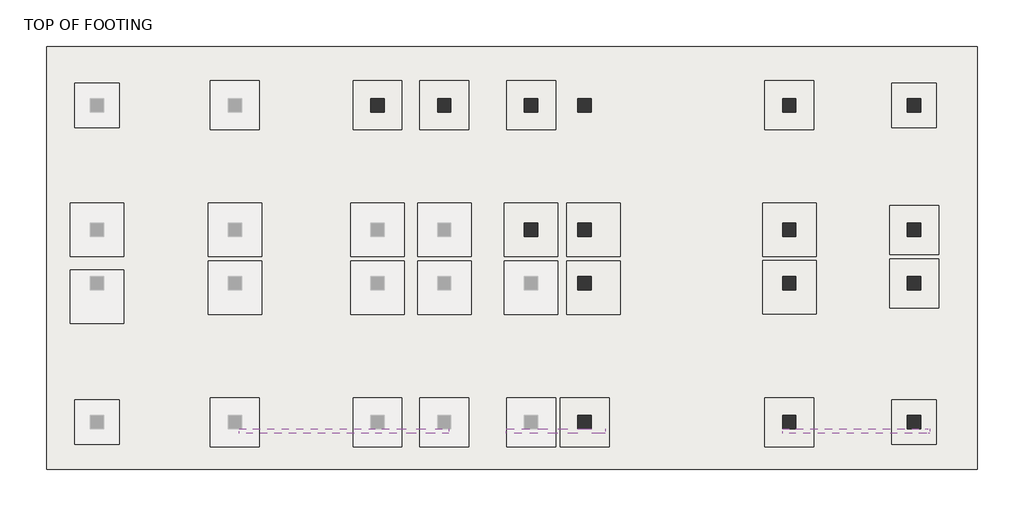
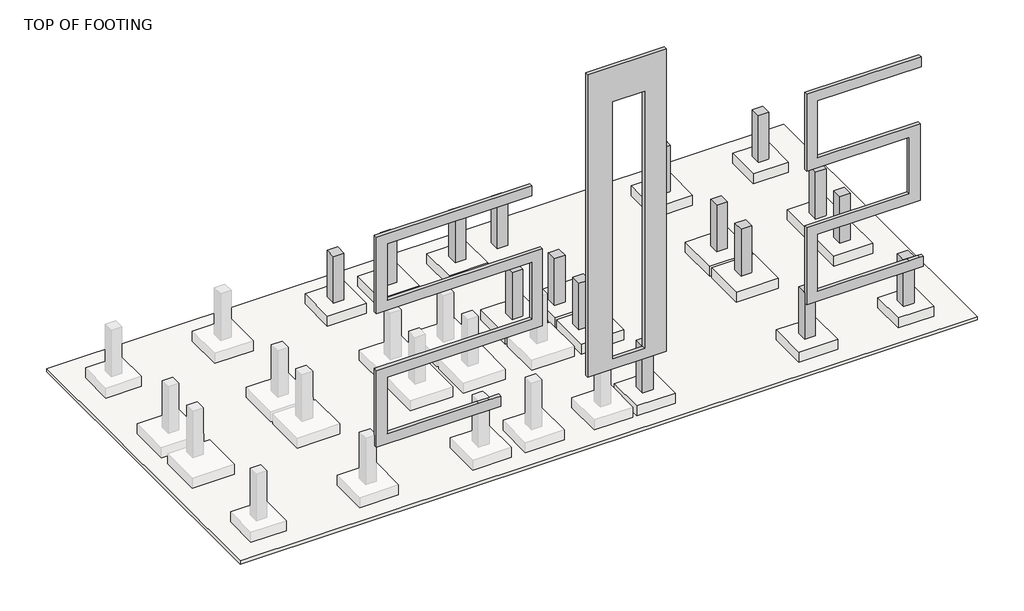
# One storey, part 2 of 2: 16 columns, 16 slabs, 3 proxies.
"""IFC4 building model written with IfcOpenShell, lengths in millimetres."""

from ifc_helpers import new_model, si_unit, frame, origin, place, context, project, spatial, polyline, outline, extrude, faceted_brep, transform, mapped, element, save
from components import generic_models_10_generic_models_5_d86a18e9, generic_models_5_generic_models_5_4128d2ba, generic_models_9_generic_models_9_a1359b20

model = new_model("IFC4")

# Units and contexts
model_context = context("Model", 3, world=origin())
ifc_project = project(units=[si_unit("LENGTHUNIT", "METRE", prefix="MILLI")], contexts=[model_context])

# Site, building, storey
site = spatial("IfcSite", under=ifc_project)
building = spatial("IfcBuilding", under=site)
storey = spatial("IfcBuildingStorey", under=building, Name="TOP OF FOOTING", Elevation=-1828.8)

# Proxies
placement = place(None, origin())
generic_models_10_generic_models_5_shape = generic_models_10_generic_models_5_d86a18e9(model_context)
element("IfcBuildingElementProxy", 1, Name="Generic Models 10 : Generic Models 5", ObjectType="Generic Models 10 : Generic Models 5", at=placement, inside=storey, context=model_context, shape_type="MappedRepresentation", body=[
    mapped(generic_models_10_generic_models_5_shape, transform((18509.5584144, 0.0, 0.0), x_axis=(1.0, 0.0, 0.0), y_axis=(0.0, 1.0, 0.0), z_axis=(0.0, 0.0, 1.0))),
])
generic_models_5_generic_models_5_shape = generic_models_5_generic_models_5_4128d2ba(model_context)
element("IfcBuildingElementProxy", 2, Name="Generic Models 5 : Generic Models 5", ObjectType="Generic Models 5 : Generic Models 5", at=placement, inside=storey, context=model_context, shape_type="MappedRepresentation", body=[
    mapped(generic_models_5_generic_models_5_shape, transform((-76.3160281, 0.0, -3.5808945), x_axis=(1.0, 0.0, 0.0), y_axis=(0.0, 1.0, 0.0), z_axis=(0.0, 0.0, 1.0))),
])
generic_models_9_generic_models_9_shape = generic_models_9_generic_models_9_a1359b20(model_context)
element("IfcBuildingElementProxy", 3, Name="Generic Models 9 : Generic Models 9", ObjectType="Generic Models 9 : Generic Models 9", at=placement, inside=storey, context=model_context, shape_type="MappedRepresentation", body=[
    mapped(generic_models_9_generic_models_9_shape, transform((0.0, 0.0, 0.0), x_axis=(1.0, 0.0, 0.0), y_axis=(0.0, 1.0, 0.0), z_axis=(0.0, 0.0, 1.0))),
])

# Columns
element("IfcColumn", 4, ObjectType="Concrete-Rectangular-Column : COLUMN 18\" X 18\"", at=placement, inside=storey, context=model_context, shape_type="SweptSolid", body=[
    extrude(outline(polyline([(-5315.5456086, 194.8205296), (-5315.5456086, -262.3794704), (-5772.7456086, -262.3794704), (-5772.7456086, 194.8205296), (-5315.5456086, 194.8205296)])), frame((0.0, 0.0, -1828.8), z_axis=(0.0, 0.0, 1.0), x_axis=(1.0, 0.0, 0.0)), (0.0, 0.0, 1.0), 2133.6),
])
element("IfcColumn", 5, ObjectType="Concrete-Rectangular-Column : COLUMN 18\" X 18\"", at=placement, inside=storey, context=model_context, shape_type="SweptSolid", body=[
    extrude(outline(polyline([(-3029.5456086, 194.8205296), (-3029.5456086, -262.3794704), (-3486.7456086, -262.3794704), (-3486.7456086, 194.8205296), (-3029.5456086, 194.8205296)])), frame((0.0, 0.0, -1828.8), z_axis=(0.0, 0.0, 1.0), x_axis=(1.0, 0.0, 0.0)), (0.0, 0.0, 1.0), 2133.6),
])
element("IfcColumn", 6, ObjectType="Concrete-Rectangular-Column : COLUMN 18\" X 18\"", at=placement, inside=storey, context=model_context, shape_type="SweptSolid", body=[
    extrude(outline(polyline([(-61.2083398, 194.8205296), (-61.2083398, -262.3794704), (-518.4083398, -262.3794704), (-518.4083398, 194.8205296), (-61.2083398, 194.8205296)])), frame((0.0, 0.0, -1828.8), z_axis=(0.0, 0.0, 1.0), x_axis=(1.0, 0.0, 0.0)), (0.0, 0.0, 1.0), 2133.6),
])
element("IfcColumn", 7, ObjectType="Concrete-Rectangular-Column : COLUMN 18\" X 18\"", at=placement, inside=storey, context=model_context, shape_type="SweptSolid", body=[
    extrude(outline(polyline([(1767.5916602, 194.8205296), (1767.5916602, -262.3794704), (1310.3916602, -262.3794704), (1310.3916602, 194.8205296), (1767.5916602, 194.8205296)])), frame((0.0, 0.0, -1828.8), z_axis=(0.0, 0.0, 1.0), x_axis=(1.0, 0.0, 0.0)), (0.0, 0.0, 1.0), 2133.6),
])
element("IfcColumn", 8, ObjectType="Concrete-Rectangular-Column : COLUMN 18\" X 18\"", at=placement, inside=storey, context=model_context, shape_type="SweptSolid", body=[
    extrude(outline(polyline([(8774.4128058, 194.8205296), (8774.4128058, -262.3794704), (8317.2128058, -262.3794704), (8317.2128058, 194.8205296), (8774.4128058, 194.8205296)])), frame((0.0, 0.0, -1828.8), z_axis=(0.0, 0.0, 1.0), x_axis=(1.0, 0.0, 0.0)), (0.0, 0.0, 1.0), 2133.6),
])
element("IfcColumn", 9, ObjectType="Concrete-Rectangular-Column : COLUMN 18\" X 18\"", at=placement, inside=storey, context=model_context, shape_type="SweptSolid", body=[
    extrude(outline(polyline([(13041.6128058, 194.8205296), (13041.6128058, -262.3794704), (12584.4128058, -262.3794704), (12584.4128058, 194.8205296), (13041.6128058, 194.8205296)])), frame((0.0, 0.0, -1828.8), z_axis=(0.0, 0.0, 1.0), x_axis=(1.0, 0.0, 0.0)), (0.0, 0.0, 1.0), 2133.6),
])
element("IfcColumn", 10, ObjectType="Concrete-Rectangular-Column : COLUMN 18\" X 18\"", at=placement, inside=storey, context=model_context, shape_type="SweptSolid", body=[
    extrude(outline(polyline([(13041.6128058, -4072.3794704), (13041.6128058, -4529.5794704), (12584.4128058, -4529.5794704), (12584.4128058, -4072.3794704), (13041.6128058, -4072.3794704)])), frame((0.0, 0.0, -1828.8), z_axis=(0.0, 0.0, 1.0), x_axis=(1.0, 0.0, 0.0)), (0.0, 0.0, 1.0), 2133.6),
])
element("IfcColumn", 11, ObjectType="Concrete-Rectangular-Column : COLUMN 18\" X 18\"", at=placement, inside=storey, context=model_context, shape_type="SweptSolid", body=[
    extrude(outline(polyline([(13041.6128058, -5901.1794704), (13041.6128058, -6358.3794704), (12584.4128058, -6358.3794704), (12584.4128058, -5901.1794704), (13041.6128058, -5901.1794704)])), frame((0.0, 0.0, -1828.8), z_axis=(0.0, 0.0, 1.0), x_axis=(1.0, 0.0, 0.0)), (0.0, 0.0, 1.0), 2133.6),
])
element("IfcColumn", 12, ObjectType="Concrete-Rectangular-Column : COLUMN 18\" X 18\"", at=placement, inside=storey, context=model_context, shape_type="SweptSolid", body=[
    extrude(outline(polyline([(13041.6128058, -10659.2679047), (13041.6128058, -11116.4679047), (12584.4128058, -11116.4679047), (12584.4128058, -10659.2679047), (13041.6128058, -10659.2679047)])), frame((0.0, 0.0, -1828.8), z_axis=(0.0, 0.0, 1.0), x_axis=(1.0, 0.0, 0.0)), (0.0, 0.0, 1.0), 2133.6),
])
element("IfcColumn", 13, ObjectType="Concrete-Rectangular-Column : COLUMN 18\" X 18\"", at=placement, inside=storey, context=model_context, shape_type="SweptSolid", body=[
    extrude(outline(polyline([(8774.4128058, -10659.2679047), (8774.4128058, -11116.4679047), (8317.2128058, -11116.4679047), (8317.2128058, -10659.2679047), (8774.4128058, -10659.2679047)])), frame((0.0, 0.0, -1828.8), z_axis=(0.0, 0.0, 1.0), x_axis=(1.0, 0.0, 0.0)), (0.0, 0.0, 1.0), 2133.6),
])
element("IfcColumn", 14, ObjectType="Concrete-Rectangular-Column : COLUMN 18\" X 18\"", at=placement, inside=storey, context=model_context, shape_type="SweptSolid", body=[
    extrude(outline(polyline([(1767.5916602, -10659.2679047), (1767.5916602, -11116.4679047), (1310.3916602, -11116.4679047), (1310.3916602, -10659.2679047), (1767.5916602, -10659.2679047)])), frame((0.0, 0.0, -1828.8), z_axis=(0.0, 0.0, 1.0), x_axis=(1.0, 0.0, 0.0)), (0.0, 0.0, 1.0), 2133.6),
])
element("IfcColumn", 15, ObjectType="Concrete-Rectangular-Column : COLUMN 18\" X 18\"", at=placement, inside=storey, context=model_context, shape_type="Brep", body=[
    faceted_brep([(-61.2083398, -4072.3794704, -1828.8), (-61.2083398, -4529.5794704, -1828.8), (-518.4083398, -4529.5794704, -1828.8), (-518.4083398, -4072.3794704, -1828.8), (-61.2083398, -4072.3794704, 152.4), (-61.2083398, -4072.3794704, 304.8), (-61.2083398, -4529.5794704, 304.8), (-61.2083398, -4529.5794704, 152.4), (-518.4083398, -4529.5794704, 304.8), (-518.4083398, -4529.5794704, 152.4), (-518.4083398, -4072.3794704, 304.8)], [[[0, 1, 2, 3]], [[1, 0, 4, 5, 6, 7]], [[2, 1, 7, 6, 8, 9]], [[3, 2, 9, 8, 10]], [[0, 3, 10, 5, 4]], [[6, 5, 10, 8]]]),
])
element("IfcColumn", 16, ObjectType="Concrete-Rectangular-Column : COLUMN 18\" X 18\"", at=placement, inside=storey, context=model_context, shape_type="Brep", body=[
    faceted_brep([(1767.5916602, -4072.3794704, -1828.8), (1767.5916602, -4529.5794704, -1828.8), (1310.3916602, -4529.5794704, -1828.8), (1310.3916602, -4072.3794704, -1828.8), (1767.5916602, -4072.3794704, 304.8), (1767.5916602, -4529.5794704, 304.8), (1767.5916602, -4529.5794704, 152.4), (1310.3916602, -4529.5794704, 304.8), (1310.3916602, -4529.5794704, 152.4), (1310.3916602, -4072.3794704, 304.8), (1310.3916602, -4072.3794704, 152.4), (1399.2916602, -4072.3794704, 304.8)], [[[0, 1, 2, 3]], [[1, 0, 4, 5, 6]], [[2, 1, 6, 5, 7, 8]], [[3, 2, 8, 7, 9, 10]], [[0, 3, 10, 9, 11, 4]], [[5, 4, 11, 9, 7]]]),
])
element("IfcColumn", 17, ObjectType="Concrete-Rectangular-Column : COLUMN 18\" X 18\"", at=placement, inside=storey, context=model_context, shape_type="Brep", body=[
    faceted_brep([(8774.4128058, -4072.3794704, -1828.8), (8774.4128058, -4529.5794704, -1828.8), (8317.2128058, -4529.5794704, -1828.8), (8317.2128058, -4072.3794704, -1828.8), (8774.4128058, -4072.3794704, 304.8), (8774.4128058, -4529.5794704, 304.8), (8774.4128058, -4529.5794704, 152.4), (8317.2128058, -4529.5794704, 304.8), (8317.2128058, -4529.5794704, 152.4), (8317.2128058, -4072.3794704, 304.8)], [[[0, 1, 2, 3]], [[1, 0, 4, 5, 6]], [[2, 1, 6, 5, 7, 8]], [[3, 2, 8, 7, 9]], [[0, 3, 9, 4]], [[5, 4, 9, 7]]]),
])
element("IfcColumn", 18, ObjectType="Concrete-Rectangular-Column : COLUMN 18\" X 18\"", at=placement, inside=storey, context=model_context, shape_type="Brep", body=[
    faceted_brep([(8774.4128058, -5901.1794704, -1828.8), (8774.4128058, -6358.3794704, -1828.8), (8317.2128058, -6358.3794704, -1828.8), (8317.2128058, -5901.1794704, -1828.8), (8774.4128058, -5901.1794704, 152.4), (8774.4128058, -5901.1794704, 304.8), (8774.4128058, -6358.3794704, 304.8), (8317.2128058, -6358.3794704, 304.8), (8317.2128058, -5901.1794704, 304.8), (8317.2128058, -5901.1794704, 152.4)], [[[0, 1, 2, 3]], [[1, 0, 4, 5, 6]], [[2, 1, 6, 7]], [[3, 2, 7, 8, 9]], [[0, 3, 9, 8, 5, 4]], [[6, 5, 8, 7]]]),
])
element("IfcColumn", 19, ObjectType="Concrete-Rectangular-Column : COLUMN 18\" X 18\"", at=placement, inside=storey, context=model_context, shape_type="Brep", body=[
    faceted_brep([(1767.5916602, -5901.1794704, -1828.8), (1767.5916602, -6358.3794704, -1828.8), (1310.3916602, -6358.3794704, -1828.8), (1310.3916602, -5901.1794704, -1828.8), (1767.5916602, -5901.1794704, 152.4), (1767.5916602, -5901.1794704, 304.8), (1767.5916602, -6358.3794704, 304.8), (1767.5916602, -6358.3794704, 152.4), (1589.7916602, -6358.3794704, 304.8), (1310.3916602, -6358.3794704, 304.8), (1310.3916602, -5901.1794704, 304.8), (1310.3916602, -5901.1794704, 152.4)], [[[0, 1, 2, 3]], [[1, 0, 4, 5, 6, 7]], [[2, 1, 7, 6, 8, 9]], [[3, 2, 9, 10, 11]], [[0, 3, 11, 10, 5, 4]], [[6, 5, 10, 9, 8]]]),
])

# Slabs
element("IfcSlab", 20, ObjectType="6\" Foundation Slab", at=placement, inside=storey, context=model_context, shape_type="Brep", body=[
    faceted_brep([(14983.6583879, 1982.0199857, -2438.4), (14983.6583879, -12495.9800143, -2438.4), (-16867.9416121, -12495.9800143, -2438.4), (-16867.9416121, 1982.0199857, -2438.4), (-14383.3456086, -10125.8679047, -2438.4), (-15907.3456086, -10125.8679047, -2438.4), (-15907.3456086, -11649.8679047, -2438.4), (-14383.3456086, -11649.8679047, -2438.4), (-9582.7456086, -10049.6679047, -2438.4), (-11259.1456086, -10049.6679047, -2438.4), (-11259.1456086, -11726.0679047, -2438.4), (-9582.7456086, -11726.0679047, -2438.4), (-4705.9456086, -10049.6679047, -2438.4), (-6382.3456086, -10049.6679047, -2438.4), (-6382.3456086, -11726.0679047, -2438.4), (-4705.9456086, -11726.0679047, -2438.4), (-2419.9456086, -10049.6679047, -2438.4), (-4096.3456086, -10049.6679047, -2438.4), (-4096.3456086, -11726.0679047, -2438.4), (-2419.9456086, -11726.0679047, -2438.4), (548.3916602, -10049.6679047, -2438.4), (-1128.0083398, -10049.6679047, -2438.4), (-1128.0083398, -11726.0679047, -2438.4), (548.3916602, -11726.0679047, -2438.4), (2377.1916602, -10049.6679047, -2438.4), (700.7916602, -10049.6679047, -2438.4), (700.7916602, -11726.0679047, -2438.4), (2377.1916602, -11726.0679047, -2438.4), (9384.0128058, -10049.6679047, -2438.4), (7707.6128058, -10049.6679047, -2438.4), (7707.6128058, -11726.0679047, -2438.4), (9384.0128058, -11726.0679047, -2438.4), (13575.0128058, -10125.8679047, -2438.4), (12051.0128058, -10125.8679047, -2438.4), (12051.0128058, -11649.8679047, -2438.4), (13575.0128058, -11649.8679047, -2438.4), (13651.2128058, -5291.5794704, -2438.4), (11974.8128058, -5291.5794704, -2438.4), (11974.8128058, -6967.9794704, -2438.4), (13651.2128058, -6967.9794704, -2438.4), (13651.2128058, -3462.7794704, -2438.4), (11974.8128058, -3462.7794704, -2438.4), (11974.8128058, -5139.1794704, -2438.4), (13651.2128058, -5139.1794704, -2438.4), (-14383.3456086, 728.2205296, -2438.4), (-15907.3456086, 728.2205296, -2438.4), (-15907.3456086, -795.7794704, -2438.4), (-14383.3456086, -795.7794704, -2438.4), (-9582.7456086, 804.4205296, -2438.4), (-11259.1456086, 804.4205296, -2438.4), (-11259.1456086, -871.9794704, -2438.4), (-9582.7456086, -871.9794704, -2438.4), (-4705.9456086, 804.4205296, -2438.4), (-6382.3456086, 804.4205296, -2438.4), (-6382.3456086, -871.9794704, -2438.4), (-4705.9456086, -871.9794704, -2438.4), (-2419.9456086, 804.4205296, -2438.4), (-4096.3456086, 804.4205296, -2438.4), (-4096.3456086, -871.9794704, -2438.4), (-2419.9456086, -871.9794704, -2438.4), (548.3916602, 804.4205296, -2438.4), (-1128.0083398, 804.4205296, -2438.4), (-1128.0083398, -871.9794704, -2438.4), (548.3916602, -871.9794704, -2438.4), (9384.0128058, 804.4205296, -2438.4), (7707.6128058, 804.4205296, -2438.4), (7707.6128058, -871.9794704, -2438.4), (9384.0128058, -871.9794704, -2438.4), (13575.0128058, 728.2205296, -2438.4), (12051.0128058, 728.2205296, -2438.4), (12051.0128058, -795.7794704, -2438.4), (13575.0128058, -795.7794704, -2438.4), (-14230.9456086, -3386.5794704, -2438.4), (-16059.7456086, -3386.5794704, -2438.4), (-16059.7456086, -5215.3794704, -2438.4), (-14230.9456086, -5215.3794704, -2438.4), (-14230.9456086, -5672.5794704, -2438.4), (-16059.7456086, -5672.5794704, -2438.4), (-16059.7456086, -7501.3794704, -2438.4), (-14230.9456086, -7501.3794704, -2438.4), (-9506.5456086, -3386.5794704, -2438.4), (-11335.3456086, -3386.5794704, -2438.4), (-11335.3456086, -5215.3794704, -2438.4), (-9506.5456086, -5215.3794704, -2438.4), (-4629.7456086, -3386.5794704, -2438.4), (-6458.5456086, -3386.5794704, -2438.4), (-6458.5456086, -5215.3794704, -2438.4), (-4629.7456086, -5215.3794704, -2438.4), (-2343.7456086, -3386.5794704, -2438.4), (-4172.5456086, -3386.5794704, -2438.4), (-4172.5456086, -5215.3794704, -2438.4), (-2343.7456086, -5215.3794704, -2438.4), (624.5916602, -3386.5794704, -2438.4), (-1204.2083398, -3386.5794704, -2438.4), (-1204.2083398, -5215.3794704, -2438.4), (624.5916602, -5215.3794704, -2438.4), (2754.6128058, -3386.5794704, -2438.4), (925.8128058, -3386.5794704, -2438.4), (925.8128058, -5215.3794704, -2438.4), (2754.6128058, -5215.3794704, -2438.4), (9460.2128058, -3386.5794704, -2438.4), (7631.4128058, -3386.5794704, -2438.4), (7631.4128058, -5215.3794704, -2438.4), (9460.2128058, -5215.3794704, -2438.4), (9460.2128058, -5342.3794704, -2438.4), (7631.4128058, -5342.3794704, -2438.4), (7631.4128058, -7171.1794704, -2438.4), (9460.2128058, -7171.1794704, -2438.4), (2754.6128058, -5367.7794704, -2438.4), (925.8128058, -5367.7794704, -2438.4), (925.8128058, -7196.5794704, -2438.4), (2754.6128058, -7196.5794704, -2438.4), (624.5916602, -5367.7794704, -2438.4), (-1204.2083398, -5367.7794704, -2438.4), (-1204.2083398, -7196.5794704, -2438.4), (624.5916602, -7196.5794704, -2438.4), (-2343.7456086, -5367.7794704, -2438.4), (-4172.5456086, -5367.7794704, -2438.4), (-4172.5456086, -7196.5794704, -2438.4), (-2343.7456086, -7196.5794704, -2438.4), (-4629.7456086, -5367.7794704, -2438.4), (-6458.5456086, -5367.7794704, -2438.4), (-6458.5456086, -7196.5794704, -2438.4), (-4629.7456086, -7196.5794704, -2438.4), (-9506.5456086, -5367.7794704, -2438.4), (-11335.3456086, -5367.7794704, -2438.4), (-11335.3456086, -7196.5794704, -2438.4), (-9506.5456086, -7196.5794704, -2438.4), (14983.6583879, 1982.0199857, -2286.0), (-16867.9416121, 1982.0199857, -2286.0), (-16867.9416121, -12495.9800143, -2286.0), (14983.6583879, -12495.9800143, -2286.0), (-14383.3456086, -10125.8679047, -2286.0), (-14383.3456086, -11649.8679047, -2286.0), (-15907.3456086, -11649.8679047, -2286.0), (-15907.3456086, -10125.8679047, -2286.0), (-9582.7456086, -10049.6679047, -2286.0), (-9582.7456086, -11726.0679047, -2286.0), (-11259.1456086, -11726.0679047, -2286.0), (-11259.1456086, -10049.6679047, -2286.0), (-4705.9456086, -10049.6679047, -2286.0), (-4705.9456086, -11726.0679047, -2286.0), (-6382.3456086, -11726.0679047, -2286.0), (-6382.3456086, -10049.6679047, -2286.0), (-2419.9456086, -10049.6679047, -2286.0), (-2419.9456086, -11726.0679047, -2286.0), (-4096.3456086, -11726.0679047, -2286.0), (-4096.3456086, -10049.6679047, -2286.0), (548.3916602, -10049.6679047, -2286.0), (548.3916602, -11726.0679047, -2286.0), (-1128.0083398, -11726.0679047, -2286.0), (-1128.0083398, -10049.6679047, -2286.0), (2377.1916602, -10049.6679047, -2286.0), (2377.1916602, -11726.0679047, -2286.0), (700.7916602, -11726.0679047, -2286.0), (700.7916602, -10049.6679047, -2286.0), (9384.0128058, -10049.6679047, -2286.0), (9384.0128058, -11726.0679047, -2286.0), (7707.6128058, -11726.0679047, -2286.0), (7707.6128058, -10049.6679047, -2286.0), (13575.0128058, -10125.8679047, -2286.0), (13575.0128058, -11649.8679047, -2286.0), (12051.0128058, -11649.8679047, -2286.0), (12051.0128058, -10125.8679047, -2286.0), (-14230.9456086, -5672.5794704, -2286.0), (-14230.9456086, -7501.3794704, -2286.0), (-16059.7456086, -7501.3794704, -2286.0), (-16059.7456086, -5672.5794704, -2286.0), (-9506.5456086, -5367.7794704, -2286.0), (-9506.5456086, -7196.5794704, -2286.0), (-11335.3456086, -7196.5794704, -2286.0), (-11335.3456086, -5367.7794704, -2286.0), (-4629.7456086, -5367.7794704, -2286.0), (-4629.7456086, -7196.5794704, -2286.0), (-6458.5456086, -7196.5794704, -2286.0), (-6458.5456086, -5367.7794704, -2286.0), (-2343.7456086, -5367.7794704, -2286.0), (-2343.7456086, -7196.5794704, -2286.0), (-4172.5456086, -7196.5794704, -2286.0), (-4172.5456086, -5367.7794704, -2286.0), (624.5916602, -5367.7794704, -2286.0), (624.5916602, -7196.5794704, -2286.0), (-1204.2083398, -7196.5794704, -2286.0), (-1204.2083398, -5367.7794704, -2286.0), (2754.6128058, -5367.7794704, -2286.0), (2754.6128058, -7196.5794704, -2286.0), (925.8128058, -7196.5794704, -2286.0), (925.8128058, -5367.7794704, -2286.0), (9460.2128058, -5342.3794704, -2286.0), (9460.2128058, -7171.1794704, -2286.0), (7631.4128058, -7171.1794704, -2286.0), (7631.4128058, -5342.3794704, -2286.0), (13651.2128058, -5291.5794704, -2286.0), (13651.2128058, -6967.9794704, -2286.0), (11974.8128058, -6967.9794704, -2286.0), (11974.8128058, -5291.5794704, -2286.0), (-14230.9456086, -3386.5794704, -2286.0), (-14230.9456086, -5215.3794704, -2286.0), (-16059.7456086, -5215.3794704, -2286.0), (-16059.7456086, -3386.5794704, -2286.0), (-9506.5456086, -3386.5794704, -2286.0), (-9506.5456086, -5215.3794704, -2286.0), (-11335.3456086, -5215.3794704, -2286.0), (-11335.3456086, -3386.5794704, -2286.0), (-4629.7456086, -3386.5794704, -2286.0), (-4629.7456086, -5215.3794704, -2286.0), (-6458.5456086, -5215.3794704, -2286.0), (-6458.5456086, -3386.5794704, -2286.0), (-2343.7456086, -3386.5794704, -2286.0), (-2343.7456086, -5215.3794704, -2286.0), (-4172.5456086, -5215.3794704, -2286.0), (-4172.5456086, -3386.5794704, -2286.0), (624.5916602, -3386.5794704, -2286.0), (624.5916602, -5215.3794704, -2286.0), (-1204.2083398, -5215.3794704, -2286.0), (-1204.2083398, -3386.5794704, -2286.0), (2754.6128058, -3386.5794704, -2286.0), (2754.6128058, -5215.3794704, -2286.0), (925.8128058, -5215.3794704, -2286.0), (925.8128058, -3386.5794704, -2286.0), (9460.2128058, -3386.5794704, -2286.0), (9460.2128058, -5215.3794704, -2286.0), (7631.4128058, -5215.3794704, -2286.0), (7631.4128058, -3386.5794704, -2286.0), (13651.2128058, -3462.7794704, -2286.0), (13651.2128058, -5139.1794704, -2286.0), (11974.8128058, -5139.1794704, -2286.0), (11974.8128058, -3462.7794704, -2286.0), (-14383.3456086, 728.2205296, -2286.0), (-14383.3456086, -795.7794704, -2286.0), (-15907.3456086, -795.7794704, -2286.0), (-15907.3456086, 728.2205296, -2286.0), (-9582.7456086, 804.4205296, -2286.0), (-9582.7456086, -871.9794704, -2286.0), (-11259.1456086, -871.9794704, -2286.0), (-11259.1456086, 804.4205296, -2286.0), (-4705.9456086, 804.4205296, -2286.0), (-4705.9456086, -871.9794704, -2286.0), (-6382.3456086, -871.9794704, -2286.0), (-6382.3456086, 804.4205296, -2286.0), (-2419.9456086, 804.4205296, -2286.0), (-2419.9456086, -871.9794704, -2286.0), (-4096.3456086, -871.9794704, -2286.0), (-4096.3456086, 804.4205296, -2286.0), (548.3916602, 804.4205296, -2286.0), (548.3916602, -871.9794704, -2286.0), (-1128.0083398, -871.9794704, -2286.0), (-1128.0083398, 804.4205296, -2286.0), (9384.0128058, 804.4205296, -2286.0), (9384.0128058, -871.9794704, -2286.0), (7707.6128058, -871.9794704, -2286.0), (7707.6128058, 804.4205296, -2286.0), (13575.0128058, 728.2205296, -2286.0), (13575.0128058, -795.7794704, -2286.0), (12051.0128058, -795.7794704, -2286.0), (12051.0128058, 728.2205296, -2286.0), (-14383.3456086, -10125.8679047, -2362.2), (-15907.3456086, -10125.8679047, -2362.2), (-15907.3456086, -11649.8679047, -2362.2), (-14383.3456086, -11649.8679047, -2362.2), (-9582.7456086, -10049.6679047, -2362.2), (-11259.1456086, -10049.6679047, -2362.2), (-11259.1456086, -11726.0679047, -2362.2), (-9582.7456086, -11726.0679047, -2362.2), (-4705.9456086, -10049.6679047, -2362.2), (-6382.3456086, -10049.6679047, -2362.2), (-6382.3456086, -11726.0679047, -2362.2), (-4705.9456086, -11726.0679047, -2362.2), (-2419.9456086, -10049.6679047, -2362.2), (-4096.3456086, -10049.6679047, -2362.2), (-4096.3456086, -11726.0679047, -2362.2), (-2419.9456086, -11726.0679047, -2362.2), (548.3916602, -10049.6679047, -2362.2), (-1128.0083398, -10049.6679047, -2362.2), (-1128.0083398, -11726.0679047, -2362.2), (548.3916602, -11726.0679047, -2362.2), (2377.1916602, -10049.6679047, -2362.2), (700.7916602, -10049.6679047, -2362.2), (700.7916602, -11726.0679047, -2362.2), (2377.1916602, -11726.0679047, -2362.2), (9384.0128058, -10049.6679047, -2362.2), (7707.6128058, -10049.6679047, -2362.2), (7707.6128058, -11726.0679047, -2362.2), (9384.0128058, -11726.0679047, -2362.2), (13575.0128058, -10125.8679047, -2362.2), (12051.0128058, -10125.8679047, -2362.2), (12051.0128058, -11649.8679047, -2362.2), (13575.0128058, -11649.8679047, -2362.2), (13651.2128058, -5291.5794704, -2362.2), (11974.8128058, -5291.5794704, -2362.2), (11974.8128058, -6967.9794704, -2362.2), (13651.2128058, -6967.9794704, -2362.2), (13651.2128058, -3462.7794704, -2362.2), (11974.8128058, -3462.7794704, -2362.2), (11974.8128058, -5139.1794704, -2362.2), (13651.2128058, -5139.1794704, -2362.2), (-14383.3456086, 728.2205296, -2362.2), (-15907.3456086, 728.2205296, -2362.2), (-15907.3456086, -795.7794704, -2362.2), (-14383.3456086, -795.7794704, -2362.2), (-9582.7456086, 804.4205296, -2362.2), (-11259.1456086, 804.4205296, -2362.2), (-11259.1456086, -871.9794704, -2362.2), (-9582.7456086, -871.9794704, -2362.2), (-4705.9456086, 804.4205296, -2362.2), (-6382.3456086, 804.4205296, -2362.2), (-6382.3456086, -871.9794704, -2362.2), (-4705.9456086, -871.9794704, -2362.2), (-2419.9456086, 804.4205296, -2362.2), (-4096.3456086, 804.4205296, -2362.2), (-4096.3456086, -871.9794704, -2362.2), (-2419.9456086, -871.9794704, -2362.2), (548.3916602, 804.4205296, -2362.2), (-1128.0083398, 804.4205296, -2362.2), (-1128.0083398, -871.9794704, -2362.2), (548.3916602, -871.9794704, -2362.2), (9384.0128058, 804.4205296, -2362.2), (7707.6128058, 804.4205296, -2362.2), (7707.6128058, -871.9794704, -2362.2), (9384.0128058, -871.9794704, -2362.2), (13575.0128058, 728.2205296, -2362.2), (12051.0128058, 728.2205296, -2362.2), (12051.0128058, -795.7794704, -2362.2), (13575.0128058, -795.7794704, -2362.2)], [[[0, 1, 2, 3], [4, 5, 6, 7], [8, 9, 10, 11], [12, 13, 14, 15], [16, 17, 18, 19], [20, 21, 22, 23], [24, 25, 26, 27], [28, 29, 30, 31], [32, 33, 34, 35], [36, 37, 38, 39], [40, 41, 42, 43], [44, 45, 46, 47], [48, 49, 50, 51], [52, 53, 54, 55], [56, 57, 58, 59], [60, 61, 62, 63], [64, 65, 66, 67], [68, 69, 70, 71], [72, 73, 74, 75], [76, 77, 78, 79], [80, 81, 82, 83], [84, 85, 86, 87], [88, 89, 90, 91], [92, 93, 94, 95], [96, 97, 98, 99], [100, 101, 102, 103], [104, 105, 106, 107], [108, 109, 110, 111], [112, 113, 114, 115], [116, 117, 118, 119], [120, 121, 122, 123], [124, 125, 126, 127]], [[128, 129, 130, 131], [132, 133, 134, 135], [136, 137, 138, 139], [140, 141, 142, 143], [144, 145, 146, 147], [148, 149, 150, 151], [152, 153, 154, 155], [156, 157, 158, 159], [160, 161, 162, 163], [164, 165, 166, 167], [168, 169, 170, 171], [172, 173, 174, 175], [176, 177, 178, 179], [180, 181, 182, 183], [184, 185, 186, 187], [188, 189, 190, 191], [192, 193, 194, 195], [196, 197, 198, 199], [200, 201, 202, 203], [204, 205, 206, 207], [208, 209, 210, 211], [212, 213, 214, 215], [216, 217, 218, 219], [220, 221, 222, 223], [224, 225, 226, 227], [228, 229, 230, 231], [232, 233, 234, 235], [236, 237, 238, 239], [240, 241, 242, 243], [244, 245, 246, 247], [248, 249, 250, 251], [252, 253, 254, 255]], [[1, 0, 128, 131]], [[2, 1, 131, 130]], [[3, 2, 130, 129]], [[0, 3, 129, 128]], [[5, 4, 256, 132, 135, 257]], [[6, 5, 257, 135, 134, 258]], [[7, 6, 258, 134, 133, 259]], [[4, 7, 259, 133, 132, 256]], [[9, 8, 260, 136, 139, 261]], [[10, 9, 261, 139, 138, 262]], [[11, 10, 262, 138, 137, 263]], [[8, 11, 263, 137, 136, 260]], [[13, 12, 264, 140, 143, 265]], [[14, 13, 265, 143, 142, 266]], [[15, 14, 266, 142, 141, 267]], [[12, 15, 267, 141, 140, 264]], [[17, 16, 268, 144, 147, 269]], [[18, 17, 269, 147, 146, 270]], [[19, 18, 270, 146, 145, 271]], [[16, 19, 271, 145, 144, 268]], [[21, 20, 272, 148, 151, 273]], [[22, 21, 273, 151, 150, 274]], [[23, 22, 274, 150, 149, 275]], [[20, 23, 275, 149, 148, 272]], [[25, 24, 276, 152, 155, 277]], [[26, 25, 277, 155, 154, 278]], [[27, 26, 278, 154, 153, 279]], [[24, 27, 279, 153, 152, 276]], [[29, 28, 280, 156, 159, 281]], [[30, 29, 281, 159, 158, 282]], [[31, 30, 282, 158, 157, 283]], [[28, 31, 283, 157, 156, 280]], [[33, 32, 284, 160, 163, 285]], [[34, 33, 285, 163, 162, 286]], [[35, 34, 286, 162, 161, 287]], [[32, 35, 287, 161, 160, 284]], [[77, 76, 164, 167]], [[78, 77, 167, 166]], [[79, 78, 166, 165]], [[76, 79, 165, 164]], [[125, 124, 168, 171]], [[126, 125, 171, 170]], [[127, 126, 170, 169]], [[124, 127, 169, 168]], [[121, 120, 172, 175]], [[122, 121, 175, 174]], [[123, 122, 174, 173]], [[120, 123, 173, 172]], [[117, 116, 176, 179]], [[118, 117, 179, 178]], [[119, 118, 178, 177]], [[116, 119, 177, 176]], [[113, 112, 180, 183]], [[114, 113, 183, 182]], [[115, 114, 182, 181]], [[112, 115, 181, 180]], [[109, 108, 184, 187]], [[110, 109, 187, 186]], [[111, 110, 186, 185]], [[108, 111, 185, 184]], [[105, 104, 188, 191]], [[106, 105, 191, 190]], [[107, 106, 190, 189]], [[104, 107, 189, 188]], [[37, 36, 288, 192, 195, 289]], [[38, 37, 289, 195, 194, 290]], [[39, 38, 290, 194, 193, 291]], [[36, 39, 291, 193, 192, 288]], [[73, 72, 196, 199]], [[74, 73, 199, 198]], [[75, 74, 198, 197]], [[72, 75, 197, 196]], [[81, 80, 200, 203]], [[82, 81, 203, 202]], [[83, 82, 202, 201]], [[80, 83, 201, 200]], [[85, 84, 204, 207]], [[86, 85, 207, 206]], [[87, 86, 206, 205]], [[84, 87, 205, 204]], [[89, 88, 208, 211]], [[90, 89, 211, 210]], [[91, 90, 210, 209]], [[88, 91, 209, 208]], [[93, 92, 212, 215]], [[94, 93, 215, 214]], [[95, 94, 214, 213]], [[92, 95, 213, 212]], [[97, 96, 216, 219]], [[98, 97, 219, 218]], [[99, 98, 218, 217]], [[96, 99, 217, 216]], [[101, 100, 220, 223]], [[102, 101, 223, 222]], [[103, 102, 222, 221]], [[100, 103, 221, 220]], [[41, 40, 292, 224, 227, 293]], [[42, 41, 293, 227, 226, 294]], [[43, 42, 294, 226, 225, 295]], [[40, 43, 295, 225, 224, 292]], [[45, 44, 296, 228, 231, 297]], [[46, 45, 297, 231, 230, 298]], [[47, 46, 298, 230, 229, 299]], [[44, 47, 299, 229, 228, 296]], [[49, 48, 300, 232, 235, 301]], [[50, 49, 301, 235, 234, 302]], [[51, 50, 302, 234, 233, 303]], [[48, 51, 303, 233, 232, 300]], [[53, 52, 304, 236, 239, 305]], [[54, 53, 305, 239, 238, 306]], [[55, 54, 306, 238, 237, 307]], [[52, 55, 307, 237, 236, 304]], [[57, 56, 308, 240, 243, 309]], [[58, 57, 309, 243, 242, 310]], [[59, 58, 310, 242, 241, 311]], [[56, 59, 311, 241, 240, 308]], [[61, 60, 312, 244, 247, 313]], [[62, 61, 313, 247, 246, 314]], [[63, 62, 314, 246, 245, 315]], [[60, 63, 315, 245, 244, 312]], [[65, 64, 316, 248, 251, 317]], [[66, 65, 317, 251, 250, 318]], [[67, 66, 318, 250, 249, 319]], [[64, 67, 319, 249, 248, 316]], [[69, 68, 320, 252, 255, 321]], [[70, 69, 321, 255, 254, 322]], [[71, 70, 322, 254, 253, 323]], [[68, 71, 323, 253, 252, 320]]]),
])
element("IfcSlab", 21, ObjectType="Pile Cap-Rectangular : 5' 6\" X 5'6\" X 1'9\" EXTERIOR FOOTING", at=placement, inside=storey, context=model_context, shape_type="Brep", body=[
    faceted_brep([(-4705.9456086, 804.4205296, -1828.8), (-6382.3456086, 804.4205296, -1828.8), (-6382.3456086, -871.9794704, -1828.8), (-4705.9456086, -871.9794704, -1828.8), (-4705.9456086, 804.4205296, -2362.2), (-4705.9456086, -871.9794704, -2362.2), (-6382.3456086, -871.9794704, -2362.2), (-6382.3456086, 804.4205296, -2362.2), (-4705.9456086, 804.4205296, -2286.0), (-6382.3456086, 804.4205296, -2286.0), (-6382.3456086, -871.9794704, -2286.0), (-4705.9456086, -871.9794704, -2286.0)], [[[0, 1, 2, 3]], [[4, 5, 6, 7]], [[1, 0, 8, 4, 7, 9]], [[2, 1, 9, 7, 6, 10]], [[3, 2, 10, 6, 5, 11]], [[0, 3, 11, 5, 4, 8]]]),
])
element("IfcSlab", 22, ObjectType="Pile Cap-Rectangular : 5' 6\" X 5'6\" X 1'9\" EXTERIOR FOOTING", at=placement, inside=storey, context=model_context, shape_type="Brep", body=[
    faceted_brep([(-2419.9456086, 804.4205296, -1828.8), (-4096.3456086, 804.4205296, -1828.8), (-4096.3456086, -871.9794704, -1828.8), (-2419.9456086, -871.9794704, -1828.8), (-2419.9456086, 804.4205296, -2362.2), (-2419.9456086, -871.9794704, -2362.2), (-4096.3456086, -871.9794704, -2362.2), (-4096.3456086, 804.4205296, -2362.2), (-2419.9456086, 804.4205296, -2286.0), (-4096.3456086, 804.4205296, -2286.0), (-4096.3456086, -871.9794704, -2286.0), (-2419.9456086, -871.9794704, -2286.0)], [[[0, 1, 2, 3]], [[4, 5, 6, 7]], [[1, 0, 8, 4, 7, 9]], [[2, 1, 9, 7, 6, 10]], [[3, 2, 10, 6, 5, 11]], [[0, 3, 11, 5, 4, 8]]]),
])
element("IfcSlab", 23, ObjectType="Pile Cap-Rectangular : 5' 6\" X 5'6\" X 1'9\" EXTERIOR FOOTING", at=placement, inside=storey, context=model_context, shape_type="Brep", body=[
    faceted_brep([(548.3916602, 804.4205296, -1828.8), (-1128.0083398, 804.4205296, -1828.8), (-1128.0083398, -871.9794704, -1828.8), (548.3916602, -871.9794704, -1828.8), (548.3916602, 804.4205296, -2362.2), (548.3916602, -871.9794704, -2362.2), (-1128.0083398, -871.9794704, -2362.2), (-1128.0083398, 804.4205296, -2362.2), (548.3916602, 804.4205296, -2286.0), (-1128.0083398, 804.4205296, -2286.0), (-1128.0083398, -871.9794704, -2286.0), (548.3916602, -871.9794704, -2286.0)], [[[0, 1, 2, 3]], [[4, 5, 6, 7]], [[1, 0, 8, 4, 7, 9]], [[2, 1, 9, 7, 6, 10]], [[3, 2, 10, 6, 5, 11]], [[0, 3, 11, 5, 4, 8]]]),
])
element("IfcSlab", 24, ObjectType="Pile Cap-Rectangular : 5' 6\" X 5'6\" X 1'9\" EXTERIOR FOOTING", at=placement, inside=storey, context=model_context, shape_type="Brep", body=[
    faceted_brep([(9384.0128058, 804.4205296, -1828.8), (7707.6128058, 804.4205296, -1828.8), (7707.6128058, -871.9794704, -1828.8), (9384.0128058, -871.9794704, -1828.8), (9384.0128058, 804.4205296, -2362.2), (9384.0128058, -871.9794704, -2362.2), (7707.6128058, -871.9794704, -2362.2), (7707.6128058, 804.4205296, -2362.2), (9384.0128058, 804.4205296, -2286.0), (7707.6128058, 804.4205296, -2286.0), (7707.6128058, -871.9794704, -2286.0), (9384.0128058, -871.9794704, -2286.0)], [[[0, 1, 2, 3]], [[4, 5, 6, 7]], [[1, 0, 8, 4, 7, 9]], [[2, 1, 9, 7, 6, 10]], [[3, 2, 10, 6, 5, 11]], [[0, 3, 11, 5, 4, 8]]]),
])
element("IfcSlab", 25, ObjectType="Pile Cap-Rectangular : 5' 6\" X 5'6\" X 1'9\" EXTERIOR FOOTING", at=placement, inside=storey, context=model_context, shape_type="Brep", body=[
    faceted_brep([(2377.1916602, -10049.6679047, -1828.8), (700.7916602, -10049.6679047, -1828.8), (700.7916602, -11726.0679047, -1828.8), (2377.1916602, -11726.0679047, -1828.8), (2377.1916602, -10049.6679047, -2362.2), (2377.1916602, -11726.0679047, -2362.2), (700.7916602, -11726.0679047, -2362.2), (700.7916602, -10049.6679047, -2362.2), (2377.1916602, -10049.6679047, -2286.0), (700.7916602, -10049.6679047, -2286.0), (700.7916602, -11726.0679047, -2286.0), (2377.1916602, -11726.0679047, -2286.0)], [[[0, 1, 2, 3]], [[4, 5, 6, 7]], [[1, 0, 8, 4, 7, 9]], [[2, 1, 9, 7, 6, 10]], [[3, 2, 10, 6, 5, 11]], [[0, 3, 11, 5, 4, 8]]]),
])
element("IfcSlab", 26, ObjectType="Pile Cap-Rectangular : 5' 6\" X 5'6\" X 1'9\" EXTERIOR FOOTING", at=placement, inside=storey, context=model_context, shape_type="Brep", body=[
    faceted_brep([(9384.0128058, -10049.6679047, -1828.8), (7707.6128058, -10049.6679047, -1828.8), (7707.6128058, -11726.0679047, -1828.8), (9384.0128058, -11726.0679047, -1828.8), (9384.0128058, -10049.6679047, -2362.2), (9384.0128058, -11726.0679047, -2362.2), (7707.6128058, -11726.0679047, -2362.2), (7707.6128058, -10049.6679047, -2362.2), (9384.0128058, -10049.6679047, -2286.0), (7707.6128058, -10049.6679047, -2286.0), (7707.6128058, -11726.0679047, -2286.0), (9384.0128058, -11726.0679047, -2286.0)], [[[0, 1, 2, 3]], [[4, 5, 6, 7]], [[1, 0, 8, 4, 7, 9]], [[2, 1, 9, 7, 6, 10]], [[3, 2, 10, 6, 5, 11]], [[0, 3, 11, 5, 4, 8]]]),
])
element("IfcSlab", 27, ObjectType="Pile Cap-Rectangular : 5' 6\" X 5'6\" X 1'9\" EXTERIOR FOOTING", at=placement, inside=storey, context=model_context, shape_type="Brep", body=[
    faceted_brep([(13651.2128058, -3462.7794704, -1828.8), (11974.8128058, -3462.7794704, -1828.8), (11974.8128058, -5139.1794704, -1828.8), (13651.2128058, -5139.1794704, -1828.8), (13651.2128058, -3462.7794704, -2362.2), (13651.2128058, -5139.1794704, -2362.2), (11974.8128058, -5139.1794704, -2362.2), (11974.8128058, -3462.7794704, -2362.2), (13651.2128058, -3462.7794704, -2286.0), (11974.8128058, -3462.7794704, -2286.0), (11974.8128058, -5139.1794704, -2286.0), (13651.2128058, -5139.1794704, -2286.0)], [[[0, 1, 2, 3]], [[4, 5, 6, 7]], [[1, 0, 8, 4, 7, 9]], [[2, 1, 9, 7, 6, 10]], [[3, 2, 10, 6, 5, 11]], [[0, 3, 11, 5, 4, 8]]]),
])
element("IfcSlab", 28, ObjectType="Pile Cap-Rectangular : 5' 6\" X 5'6\" X 1'9\" EXTERIOR FOOTING", at=placement, inside=storey, context=model_context, shape_type="Brep", body=[
    faceted_brep([(13651.2128058, -5291.5794704, -1828.8), (11974.8128058, -5291.5794704, -1828.8), (11974.8128058, -6967.9794704, -1828.8), (13651.2128058, -6967.9794704, -1828.8), (13651.2128058, -5291.5794704, -2362.2), (13651.2128058, -6967.9794704, -2362.2), (11974.8128058, -6967.9794704, -2362.2), (11974.8128058, -5291.5794704, -2362.2), (13651.2128058, -5291.5794704, -2286.0), (11974.8128058, -5291.5794704, -2286.0), (11974.8128058, -6967.9794704, -2286.0), (13651.2128058, -6967.9794704, -2286.0)], [[[0, 1, 2, 3]], [[4, 5, 6, 7]], [[1, 0, 8, 4, 7, 9]], [[2, 1, 9, 7, 6, 10]], [[3, 2, 10, 6, 5, 11]], [[0, 3, 11, 5, 4, 8]]]),
])
element("IfcSlab", 29, ObjectType="Pile Cap-Rectangular : 5' X 5' X 1'9\" CORNER FOOTING", at=placement, inside=storey, context=model_context, shape_type="Brep", body=[
    faceted_brep([(13575.0128058, 728.2205296, -1828.8), (12051.0128058, 728.2205296, -1828.8), (12051.0128058, -795.7794704, -1828.8), (13575.0128058, -795.7794704, -1828.8), (13575.0128058, 728.2205296, -2362.2), (13575.0128058, -795.7794704, -2362.2), (12051.0128058, -795.7794704, -2362.2), (12051.0128058, 728.2205296, -2362.2), (13575.0128058, 728.2205296, -2286.0), (12051.0128058, 728.2205296, -2286.0), (12051.0128058, -795.7794704, -2286.0), (13575.0128058, -795.7794704, -2286.0)], [[[0, 1, 2, 3]], [[4, 5, 6, 7]], [[1, 0, 8, 4, 7, 9]], [[2, 1, 9, 7, 6, 10]], [[3, 2, 10, 6, 5, 11]], [[0, 3, 11, 5, 4, 8]]]),
])
element("IfcSlab", 30, ObjectType="Pile Cap-Rectangular : 5' X 5' X 1'9\" CORNER FOOTING", at=placement, inside=storey, context=model_context, shape_type="Brep", body=[
    faceted_brep([(13575.0128058, -10125.8679047, -1828.8), (12051.0128058, -10125.8679047, -1828.8), (12051.0128058, -11649.8679047, -1828.8), (13575.0128058, -11649.8679047, -1828.8), (13575.0128058, -10125.8679047, -2362.2), (13575.0128058, -11649.8679047, -2362.2), (12051.0128058, -11649.8679047, -2362.2), (12051.0128058, -10125.8679047, -2362.2), (13575.0128058, -10125.8679047, -2286.0), (12051.0128058, -10125.8679047, -2286.0), (12051.0128058, -11649.8679047, -2286.0), (13575.0128058, -11649.8679047, -2286.0)], [[[0, 1, 2, 3]], [[4, 5, 6, 7]], [[1, 0, 8, 4, 7, 9]], [[2, 1, 9, 7, 6, 10]], [[3, 2, 10, 6, 5, 11]], [[0, 3, 11, 5, 4, 8]]]),
])
element("IfcSlab", 31, ObjectType="Pile Cap-Rectangular : 6' X 6' X 2' FOOTING INTERIOR", at=placement, inside=storey, context=model_context, shape_type="Brep", body=[
    faceted_brep([(624.5916602, -3386.5794704, -1828.8), (-1204.2083398, -3386.5794704, -1828.8), (-1204.2083398, -5215.3794704, -1828.8), (624.5916602, -5215.3794704, -1828.8), (624.5916602, -3386.5794704, -2438.4), (624.5916602, -5215.3794704, -2438.4), (-1204.2083398, -5215.3794704, -2438.4), (-1204.2083398, -3386.5794704, -2438.4), (624.5916602, -3386.5794704, -2286.0), (-1204.2083398, -3386.5794704, -2286.0), (-1204.2083398, -5215.3794704, -2286.0), (624.5916602, -5215.3794704, -2286.0)], [[[0, 1, 2, 3]], [[4, 5, 6, 7]], [[1, 0, 8, 4, 7, 9]], [[2, 1, 9, 7, 6, 10]], [[3, 2, 10, 6, 5, 11]], [[0, 3, 11, 5, 4, 8]]]),
])
element("IfcSlab", 32, ObjectType="Pile Cap-Rectangular : 6' X 6' X 2' FOOTING INTERIOR", at=placement, inside=storey, context=model_context, shape_type="Brep", body=[
    faceted_brep([(2754.6128058, -3386.5794704, -1828.8), (925.8128058, -3386.5794704, -1828.8), (925.8128058, -5215.3794704, -1828.8), (2754.6128058, -5215.3794704, -1828.8), (2754.6128058, -3386.5794704, -2438.4), (2754.6128058, -5215.3794704, -2438.4), (925.8128058, -5215.3794704, -2438.4), (925.8128058, -3386.5794704, -2438.4), (2754.6128058, -3386.5794704, -2286.0), (925.8128058, -3386.5794704, -2286.0), (925.8128058, -5215.3794704, -2286.0), (2754.6128058, -5215.3794704, -2286.0)], [[[0, 1, 2, 3]], [[4, 5, 6, 7]], [[1, 0, 8, 4, 7, 9]], [[2, 1, 9, 7, 6, 10]], [[3, 2, 10, 6, 5, 11]], [[0, 3, 11, 5, 4, 8]]]),
])
element("IfcSlab", 33, ObjectType="Pile Cap-Rectangular : 6' X 6' X 2' FOOTING INTERIOR", at=placement, inside=storey, context=model_context, shape_type="Brep", body=[
    faceted_brep([(9460.2128058, -3386.5794704, -1828.8), (7631.4128058, -3386.5794704, -1828.8), (7631.4128058, -5215.3794704, -1828.8), (9460.2128058, -5215.3794704, -1828.8), (9460.2128058, -3386.5794704, -2438.4), (9460.2128058, -5215.3794704, -2438.4), (7631.4128058, -5215.3794704, -2438.4), (7631.4128058, -3386.5794704, -2438.4), (9460.2128058, -3386.5794704, -2286.0), (7631.4128058, -3386.5794704, -2286.0), (7631.4128058, -5215.3794704, -2286.0), (9460.2128058, -5215.3794704, -2286.0)], [[[0, 1, 2, 3]], [[4, 5, 6, 7]], [[1, 0, 8, 4, 7, 9]], [[2, 1, 9, 7, 6, 10]], [[3, 2, 10, 6, 5, 11]], [[0, 3, 11, 5, 4, 8]]]),
])
element("IfcSlab", 34, ObjectType="Pile Cap-Rectangular : 6' X 6' X 2' FOOTING INTERIOR", at=placement, inside=storey, context=model_context, shape_type="Brep", body=[
    faceted_brep([(9460.2128058, -5342.3794704, -1828.8), (7631.4128058, -5342.3794704, -1828.8), (7631.4128058, -7171.1794704, -1828.8), (9460.2128058, -7171.1794704, -1828.8), (9460.2128058, -5342.3794704, -2438.4), (9460.2128058, -7171.1794704, -2438.4), (7631.4128058, -7171.1794704, -2438.4), (7631.4128058, -5342.3794704, -2438.4), (9460.2128058, -5342.3794704, -2286.0), (7631.4128058, -5342.3794704, -2286.0), (7631.4128058, -7171.1794704, -2286.0), (9460.2128058, -7171.1794704, -2286.0)], [[[0, 1, 2, 3]], [[4, 5, 6, 7]], [[1, 0, 8, 4, 7, 9]], [[2, 1, 9, 7, 6, 10]], [[3, 2, 10, 6, 5, 11]], [[0, 3, 11, 5, 4, 8]]]),
])
element("IfcSlab", 35, ObjectType="Pile Cap-Rectangular : 6' X 6' X 2' FOOTING INTERIOR", at=placement, inside=storey, context=model_context, shape_type="Brep", body=[
    faceted_brep([(2754.6128058, -5367.7794704, -1828.8), (925.8128058, -5367.7794704, -1828.8), (925.8128058, -7196.5794704, -1828.8), (2754.6128058, -7196.5794704, -1828.8), (2754.6128058, -5367.7794704, -2438.4), (2754.6128058, -7196.5794704, -2438.4), (925.8128058, -7196.5794704, -2438.4), (925.8128058, -5367.7794704, -2438.4), (2754.6128058, -5367.7794704, -2286.0), (925.8128058, -5367.7794704, -2286.0), (925.8128058, -7196.5794704, -2286.0), (2754.6128058, -7196.5794704, -2286.0)], [[[0, 1, 2, 3]], [[4, 5, 6, 7]], [[1, 0, 8, 4, 7, 9]], [[2, 1, 9, 7, 6, 10]], [[3, 2, 10, 6, 5, 11]], [[0, 3, 11, 5, 4, 8]]]),
])

save(model, "model.ifc")

# Revit data of these elements
# Type "Concrete-Rectangular-Column : COLUMN 18\" X 18\""
#   Assembly Code = "B10"
#   b = 1' - 6"
#   h = 1' - 6"
#   Structural Material [instance default] = Concrete, Cast-in-Place gray
# Type "6\" Foundation Slab"
#   Layers, outside or top first: 0' - 6" "Concrete, Cast-in-Place gray" (function 1)
# Type "Pile Cap-Rectangular : 5' 6\" X 5'6\" X 1'9\" EXTERIOR FOOTING"
#   Assembly Code = "A1010100"
#   Width = 5' - 6"
#   Length = 5' - 6"
#   Foundation Thickness = 1' - 9"
#   Structural Material [instance default] = Concrete, Cast-in-Place gray
# Type "Pile Cap-Rectangular : 5' X 5' X 1'9\" CORNER FOOTING"
#   Assembly Code = "A1010100"
#   Width = 5' - 0"
#   Length = 5' - 0"
#   Foundation Thickness = 1' - 9"
#   Structural Material [instance default] = Concrete, Cast-in-Place gray
# Type "Pile Cap-Rectangular : 6' X 6' X 2' FOOTING INTERIOR"
#   Assembly Code = "A1010100"
#   Width = 6' - 0"
#   Length = 6' - 0"
#   Foundation Thickness = 2' - 0"
#   Structural Material [instance default] = Concrete, Cast-in-Place gray
# Element 1 (IfcBuildingElementProxy, "Generic Models 10 : Generic Models 5")
#   Phase Created = New Construction
#   Materials on its faces: "WALL ACCENT 6\""
# Element 2 (IfcBuildingElementProxy, "Generic Models 5 : Generic Models 5")
#   Phase Created = New Construction
#   Materials on its faces: "WALL ACCENT 6\""
# Element 3 (IfcBuildingElementProxy, "Generic Models 9 : Generic Models 9")
#   Phase Created = New Construction
#   Materials on its faces: "TEAK BROWN COLOUR"
# Elements 4, 5, 6, 7, 8, 9, 10, 11, 12, 13, 14, 15, 16, 17, 18, 19 (IfcColumn, "Concrete-Rectangular-Column : COLUMN 18\" X 18\"")
#   Structural Material = Concrete, Cast-in-Place gray
#   Phase Created = New Construction
#   Materials on its faces: "Concrete, Cast-in-Place gray"
# Element 20 (IfcSlab, "6\" Foundation Slab")
#   Height Offset From Level = -1' - 6"
#   built-in parameter 1001954 = 1
#   Phase Created = New Construction
#   Materials on its faces: "Concrete, Cast-in-Place gray"
# Elements 21, 22, 23, 24, 25, 26, 27, 28 (IfcSlab, "Pile Cap-Rectangular : 5' 6\" X 5'6\" X 1'9\" EXTERIOR FOOTING")
#   Structural Material = Concrete, Cast-in-Place gray
#   Phase Created = New Construction
#   Materials on its faces: "Concrete, Cast-in-Place gray"
# Elements 29, 30 (IfcSlab, "Pile Cap-Rectangular : 5' X 5' X 1'9\" CORNER FOOTING")
#   Structural Material = Concrete, Cast-in-Place gray
#   Phase Created = New Construction
#   Materials on its faces: "Concrete, Cast-in-Place gray"
# Elements 31, 32, 33, 34, 35 (IfcSlab, "Pile Cap-Rectangular : 6' X 6' X 2' FOOTING INTERIOR")
#   Structural Material = Concrete, Cast-in-Place gray
#   Phase Created = New Construction
#   Materials on its faces: "Concrete, Cast-in-Place gray"
# Materials
#   "Concrete, Cast-in-Place gray": class "Concrete", colour RGB 192 192 192, transparency 0, Description = "Cast-in-place concrete", Cost = 0
#   "WALL ACCENT 6\"": class "Generic", colour RGB 120 120 120, transparency 0, Cost = 0
#   "TEAK BROWN COLOUR": class "Generic", colour RGB 120 120 120, transparency 0, Cost = 0
